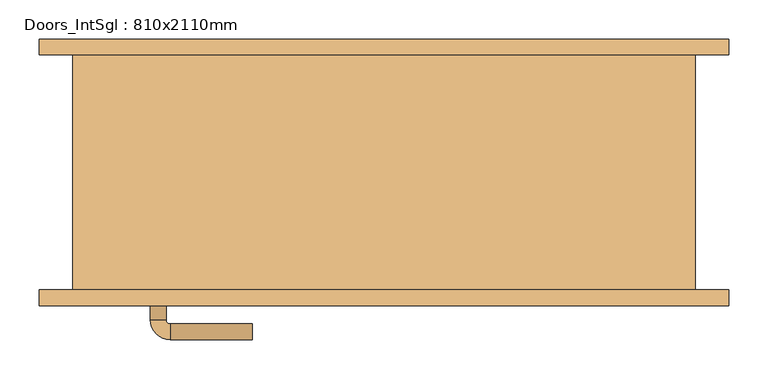
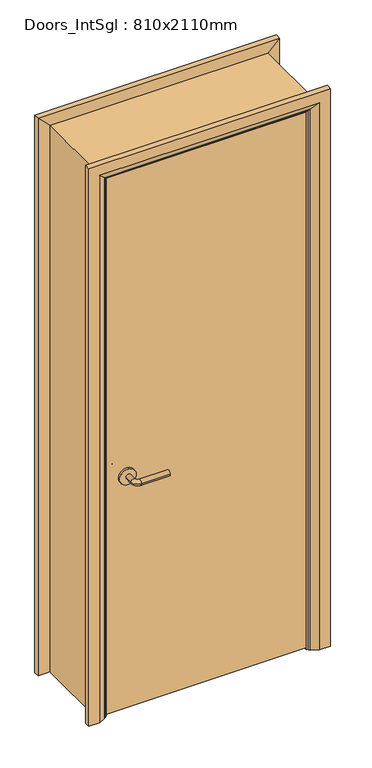
"""IFC4 building model written with IfcOpenShell, lengths in millimetres: door geometry, Doors_IntSgl : 810x2110mm."""

from ifc_helpers import new_model, si_unit, point, frame, frame_2d, origin, place, context, project, spatial, polyline, circle_curve, ellipse_curve, trimmed, segment, composite_curve, outline, extrude, faceted_brep, source, transform, mapped, element, save
from ifc_brep_helpers import plane_surface, cylinder_surface, revolved_surface, advanced_brep


def doors_intsgl_810x2110mm_8206dd41(model_context):
    return source(origin(), model_context, "Body", "SolidModel", [
        advanced_brep(
        [(-298.0, -104.0, 900.0), (-278.0, -104.0, 900.0), (-298.0, -74.0, 900.0), (-278.0, -74.0, 900.0), (-273.0, -69.0, 900.0), (-273.0, -49.0, 900.0), (-168.0, -49.0, 900.0), (-168.0, -69.0, 900.0)],
        [
            (0, 1, circle_curve(frame((-288.0, -104.0, 900.0), z_axis=(0.0, -1.0, 0.0), x_axis=(1.0, 0.0, 0.0)), 10.0)),
            (1, 0, circle_curve(frame((-288.0, -104.0, 900.0), z_axis=(0.0, -1.0, 0.0), x_axis=(1.0, 0.0, 0.0)), 10.0)),
            (0, 2),
            (2, 3, circle_curve(frame((-288.0, -74.0, 900.0), z_axis=(0.0, -1.0, 0.0), x_axis=(1.0, 0.0, 0.0)), 10.0)),
            (3, 1),
            (3, 2, circle_curve(frame((-288.0, -74.0, 900.0), z_axis=(0.0, -1.0, 0.0), x_axis=(1.0, 0.0, 0.0)), 10.0)),
            (4, 3, circle_curve(frame((-273.0, -74.0, 900.0), z_axis=(0.0, 0.0, 1.0), x_axis=(-1.0, 0.0, 0.0)), 5.0)),
            (2, 5, circle_curve(frame((-273.0, -74.0, 900.0), z_axis=(0.0, 0.0, -1.0), x_axis=(-1.0, 0.0, 0.0)), 25.0)),
            (5, 4, circle_curve(frame((-273.0, -59.0, 900.0), z_axis=(-1.0, 0.0, 0.0), x_axis=(0.0, -1.0, 0.0)), 10.0)),
            (4, 5, circle_curve(frame((-273.0, -59.0, 900.0), z_axis=(-1.0, 0.0, 0.0), x_axis=(0.0, -1.0, 0.0)), 10.0)),
            (6, 7, circle_curve(frame((-168.0, -59.0, 900.0), z_axis=(1.0, 0.0, 0.0), x_axis=(0.0, -1.0, 0.0)), 10.0)),
            (7, 6, circle_curve(frame((-168.0, -59.0, 900.0), z_axis=(1.0, 0.0, 0.0), x_axis=(0.0, -1.0, 0.0)), 10.0)),
            (5, 6),
            (7, 4),
        ],
        [
            plane_surface(frame((-288.0, -104.0, 900.0), z_axis=(0.0, -1.0, 0.0), x_axis=(0.0, 0.0, 1.0))),
            cylinder_surface(frame((-288.0, -104.0, 900.0), z_axis=(0.0, -1.0, 0.0), x_axis=(1.0, 0.0, 0.0)), 10.0),
            revolved_surface(trimmed(ellipse_curve(frame((-288.0, -74.0, 900.0), z_axis=(0.0, -1.0, 0.0), x_axis=(1.0, 0.0, 0.0)), 10.0, 10.0), [point((-298.0, -74.0, 900.0))], [point((-278.0, -74.0, 900.0))], True, "CARTESIAN"), (-273.0, -74.0, 900.0), (0.0, 0.0, -1.0)),
            revolved_surface(trimmed(ellipse_curve(frame((-288.0, -74.0, 900.0), z_axis=(0.0, -1.0, 0.0), x_axis=(1.0, 0.0, 0.0)), 10.0, 10.0), [point((-278.0, -74.0, 900.0))], [point((-298.0, -74.0, 900.0))], True, "CARTESIAN"), (-273.0, -74.0, 900.0), (0.0, 0.0, -1.0)),
            plane_surface(frame((-168.0, -59.0, 900.0), z_axis=(1.0, 0.0, 0.0), x_axis=(0.0, 0.0, 1.0))),
            cylinder_surface(frame((-273.0, -59.0, 900.0), z_axis=(-1.0, 0.0, 0.0), x_axis=(0.0, -1.0, 0.0)), 10.0),
        ],
        [
            (0, [[1, 2]]),
            (1, [[-1, 3, 4, 5]]),
            (1, [[-2, -5, 6, -3]]),
            (2, [[7, -4, 8, 9]]),
            (3, [[-8, -6, -7, 10]]),
            (4, [[11, 12]]),
            (5, [[-9, 13, -12, 14]]),
            (5, [[-10, -14, -11, -13]]),
        ],
    ),
        extrude(outline(composite_curve([segment(trimmed(circle_curve(frame_2d((900.0, -290.5)), 30.0), [point((900.0, -320.5))], [point((900.0, -260.5))], False, "CARTESIAN"), True, "CONTINUOUS"), segment(trimmed(circle_curve(frame_2d((900.0, -290.5)), 30.0), [point((900.0, -260.5))], [point((900.0, -320.5))], False, "CARTESIAN"), True, "CONTINUOUS")], self_intersect=False)), frame((0.0, -112.0, 0.0), z_axis=(0.0, 1.0, 0.0), x_axis=(0.0, 0.0, 1.0)), (0.0, 0.0, 1.0), 8.0),
        advanced_brep(
        [(-298.0, -158.0, 900.0), (-278.0, -158.0, 900.0), (-278.0, -188.0, 900.0), (-298.0, -188.0, 900.0), (-273.0, -193.0, 900.0), (-273.0, -213.0, 900.0), (-168.0, -213.0, 900.0), (-168.0, -193.0, 900.0)],
        [
            (0, 1, circle_curve(frame((-288.0, -158.0, 900.0), z_axis=(0.0, 1.0, 0.0), x_axis=(1.0, 0.0, 0.0)), 10.0)),
            (1, 0, circle_curve(frame((-288.0, -158.0, 900.0), z_axis=(0.0, 1.0, 0.0), x_axis=(1.0, 0.0, 0.0)), 10.0)),
            (1, 2),
            (2, 3, circle_curve(frame((-288.0, -188.0, 900.0), z_axis=(0.0, 1.0, 0.0), x_axis=(1.0, 0.0, 0.0)), 10.0)),
            (3, 0),
            (3, 2, circle_curve(frame((-288.0, -188.0, 900.0), z_axis=(0.0, 1.0, 0.0), x_axis=(1.0, 0.0, 0.0)), 10.0)),
            (4, 5, circle_curve(frame((-273.0, -203.0, 900.0), z_axis=(-1.0, 0.0, 0.0), x_axis=(0.0, 1.0, 0.0)), 10.0)),
            (5, 3, circle_curve(frame((-273.0, -188.0, 900.0), z_axis=(0.0, 0.0, -1.0), x_axis=(-1.0, 0.0, 0.0)), 25.0)),
            (2, 4, circle_curve(frame((-273.0, -188.0, 900.0), z_axis=(0.0, 0.0, 1.0), x_axis=(-1.0, 0.0, 0.0)), 5.0)),
            (5, 4, circle_curve(frame((-273.0, -203.0, 900.0), z_axis=(-1.0, 0.0, 0.0), x_axis=(0.0, 1.0, 0.0)), 10.0)),
            (6, 7, circle_curve(frame((-168.0, -203.0, 900.0), z_axis=(1.0, 0.0, 0.0), x_axis=(0.0, 1.0, 0.0)), 10.0)),
            (7, 6, circle_curve(frame((-168.0, -203.0, 900.0), z_axis=(1.0, 0.0, 0.0), x_axis=(0.0, 1.0, 0.0)), 10.0)),
            (4, 7),
            (6, 5),
        ],
        [
            plane_surface(frame((-288.0, -158.0, 900.0), z_axis=(0.0, 1.0, 0.0), x_axis=(0.0, 0.0, 1.0))),
            cylinder_surface(frame((-288.0, -158.0, 900.0), z_axis=(0.0, 1.0, 0.0), x_axis=(1.0, 0.0, 0.0)), 10.0),
            revolved_surface(trimmed(ellipse_curve(frame((-288.0, -188.0, 900.0), z_axis=(0.0, -1.0, 0.0), x_axis=(1.0, 0.0, 0.0)), 10.0, 10.0), [point((-298.0, -188.0, 900.0))], [point((-278.0, -188.0, 900.0))], True, "CARTESIAN"), (-273.0, -188.0, 900.0), (0.0, 0.0, -1.0)),
            revolved_surface(trimmed(ellipse_curve(frame((-288.0, -188.0, 900.0), z_axis=(0.0, -1.0, 0.0), x_axis=(1.0, 0.0, 0.0)), 10.0, 10.0), [point((-278.0, -188.0, 900.0))], [point((-298.0, -188.0, 900.0))], True, "CARTESIAN"), (-273.0, -188.0, 900.0), (0.0, 0.0, -1.0)),
            plane_surface(frame((-168.0, -203.0, 900.0), z_axis=(1.0, 0.0, 0.0), x_axis=(0.0, 0.0, 1.0))),
            cylinder_surface(frame((-273.0, -203.0, 900.0), z_axis=(-1.0, 0.0, 0.0), x_axis=(0.0, 1.0, 0.0)), 10.0),
        ],
        [
            (0, [[1, 2]]),
            (1, [[3, 4, 5, -2]]),
            (1, [[-5, 6, -3, -1]]),
            (2, [[7, 8, -4, 9]]),
            (3, [[10, -9, -6, -8]]),
            (4, [[11, 12]]),
            (5, [[13, -11, 14, -7]]),
            (5, [[-14, -12, -13, -10]]),
        ],
    ),
        extrude(outline(composite_curve([segment(trimmed(circle_curve(frame_2d((900.0, -290.5)), 30.0), [point((900.0, -320.5))], [point((900.0, -260.5))], False, "CARTESIAN"), True, "CONTINUOUS"), segment(trimmed(circle_curve(frame_2d((900.0, -290.5)), 30.0), [point((900.0, -260.5))], [point((900.0, -320.5))], False, "CARTESIAN"), True, "CONTINUOUS")], self_intersect=False)), frame((0.0, -158.0, 0.0), z_axis=(0.0, 1.0, 0.0), x_axis=(0.0, 0.0, 1.0)), (0.0, 0.0, 1.0), 8.0),
        extrude(outline(polyline([(363.0, -112.0), (363.0, -150.0), (-363.0, -150.0), (-363.0, -112.0), (363.0, -112.0)])), frame((0.0, 0.0, 8.0), z_axis=(0.0, 0.0, 1.0), x_axis=(1.0, 0.0, 0.0)), (0.0, 0.0, 1.0), 2060.0),
        advanced_brep(
        [(440.0, -170.0, 0.0), (400.0, -170.0, 0.0), (374.0, -156.0, 0.0), (370.0, -150.0, 0.0), (440.0, -150.0, 0.0), (440.0, -150.0, 2145.0), (440.0, -170.0, 2145.0), (370.0, -150.0, 2075.0), (-370.0, -150.0, 2075.0), (-370.0, -150.0, 0.0), (-440.0, -150.0, 0.0), (-440.0, -150.0, 2145.0), (374.0, -156.0, 2079.0), (400.0, -170.0, 2105.0), (-440.0, -170.0, 2145.0), (-440.0, -170.0, 0.0), (-400.0, -170.0, 0.0), (-400.0, -170.0, 2105.0), (-374.0, -156.0, 2079.0), (-374.0, -156.0, 0.0)],
        [
            (0, 1),
            (1, 2),
            (2, 3, circle_curve(frame((378.0, -149.0, 0.0), z_axis=(0.0, 0.0, -1.0), x_axis=(1.0, 0.0, 0.0)), 8.0622577)),
            (3, 4),
            (4, 0),
            (4, 5),
            (5, 6),
            (6, 0),
            (3, 7),
            (7, 8),
            (8, 9),
            (9, 10),
            (10, 11),
            (11, 5),
            (2, 12),
            (12, 7, ellipse_curve(frame((378.0, -149.0, 2083.0), z_axis=(0.7071067811865475, 0.0, -0.7071067811865475), x_axis=(-0.7071067811865474, 0.0, -0.7071067811865476)), 11.4017543, 8.0622577)),
            (1, 13),
            (13, 12),
            (6, 14),
            (14, 15),
            (15, 16),
            (16, 17),
            (17, 13),
            (11, 14),
            (12, 18),
            (18, 8, ellipse_curve(frame((-378.0, -149.0, 2083.0), z_axis=(0.7071067811865475, 0.0, 0.7071067811865475), x_axis=(0.7071067811865476, 0.0, -0.7071067811865474)), 11.4017543, 8.0622577)),
            (17, 18),
            (15, 10),
            (9, 19, circle_curve(frame((-378.0, -149.0, 0.0), z_axis=(0.0, 0.0, -1.0), x_axis=(-1.0, 0.0, 0.0)), 8.0622577)),
            (19, 16),
            (18, 19),
        ],
        [
            plane_surface(frame((370.0, -150.0, 0.0), z_axis=(0.0, 0.0, -1.0), x_axis=(0.0, 1.0, 0.0))),
            plane_surface(frame((440.0, -170.0, 0.0), z_axis=(1.0, 0.0, 0.0), x_axis=(0.0, 0.0, 1.0))),
            plane_surface(frame((440.0, -150.0, 0.0), z_axis=(0.0, 1.0, 0.0), x_axis=(0.0, 0.0, 1.0))),
            cylinder_surface(frame((378.0, -149.0, 0.0), z_axis=(0.0, 0.0, -1.0), x_axis=(1.0, 0.0, 0.0)), 8.0622577),
            plane_surface(frame((374.0, -156.0, 0.0), z_axis=(-0.4740998230350126, -0.880471099922178, 0.0), x_axis=(0.0, 0.0, 1.0))),
            plane_surface(frame((400.0, -170.0, 0.0), z_axis=(0.0, -1.0, 0.0), x_axis=(0.0, 0.0, 1.0))),
            plane_surface(frame((440.0, -170.0, 2145.0), z_axis=(0.0, 0.0, 1.0), x_axis=(-1.0, 0.0, 0.0))),
            cylinder_surface(frame((370.0, -149.0, 2083.0), z_axis=(1.0, 0.0, 0.0), x_axis=(0.0, 0.0, 1.0)), 8.0622577),
            plane_surface(frame((374.0, -156.0, 2079.0), z_axis=(0.0, -0.8804710999221764, -0.4740998230350154), x_axis=(-1.0, 0.0, 0.0))),
            plane_surface(frame((-370.0, -150.0, 0.0), z_axis=(0.0, 0.0, -1.0), x_axis=(0.0, 1.0, 0.0))),
            plane_surface(frame((-440.0, -170.0, 2145.0), z_axis=(-1.0, 0.0, 0.0), x_axis=(0.0, 0.0, -1.0))),
            cylinder_surface(frame((-378.0, -149.0, 2075.0), z_axis=(0.0, 0.0, 1.0), x_axis=(-1.0, 0.0, 0.0)), 8.0622577),
            plane_surface(frame((-374.0, -156.0, 2079.0), z_axis=(0.47409982303501824, -0.8804710999221749, 0.0), x_axis=(0.0, 0.0, -1.0))),
        ],
        [
            (0, [[1, 2, 3, 4, 5]]),
            (1, [[6, 7, 8, -5]]),
            (2, [[9, 10, 11, 12, 13, 14, -6, -4]]),
            (3, [[15, 16, -9, -3]]),
            (4, [[17, 18, -15, -2]]),
            (5, [[-8, 19, 20, 21, 22, 23, -17, -1]]),
            (6, [[-14, 24, -19, -7]]),
            (7, [[25, 26, -10, -16]]),
            (8, [[-23, 27, -25, -18]]),
            (9, [[28, -12, 29, 30, -21]]),
            (10, [[-13, -28, -20, -24]]),
            (11, [[31, -29, -11, -26]]),
            (12, [[-22, -30, -31, -27]]),
        ],
    ),
        extrude(outline(polyline([(0.0, -346.0), (2051.0, -346.0), (2051.0, 346.0), (0.0, 346.0), (0.0, 365.0), (2070.0, 365.0), (2070.0, -365.0), (0.0, -365.0), (0.0, -346.0)])), frame((0.0, -110.0, 0.0), z_axis=(0.0, 1.0, 0.0), x_axis=(0.0, 0.0, 1.0)), (0.0, 0.0, 1.0), 32.0),
        advanced_brep(
        [(-440.0, 170.0, 0.0), (-400.0, 170.0, 0.0), (-374.0, 156.0, 0.0), (-370.0, 150.0, 0.0), (-440.0, 150.0, 0.0), (-440.0, 150.0, 2145.0), (-440.0, 170.0, 2145.0), (-370.0, 150.0, 2075.0), (-374.0, 156.0, 2079.0), (-400.0, 170.0, 2105.0), (440.0, 150.0, 2145.0), (440.0, 170.0, 2145.0), (370.0, 150.0, 2075.0), (374.0, 156.0, 2079.0), (400.0, 170.0, 2105.0), (440.0, 170.0, 0.0), (440.0, 150.0, 0.0), (370.0, 150.0, 0.0), (374.0, 156.0, 0.0), (400.0, 170.0, 0.0)],
        [
            (0, 1),
            (1, 2),
            (2, 3, circle_curve(frame((-378.0, 149.0, 0.0), z_axis=(0.0, 0.0, -1.0), x_axis=(-1.0, 0.0, 0.0)), 8.0622577)),
            (3, 4),
            (4, 0),
            (4, 5),
            (5, 6),
            (6, 0),
            (3, 7),
            (7, 5),
            (2, 8),
            (8, 7, ellipse_curve(frame((-378.0, 149.0, 2083.0), z_axis=(-0.7071067811865475, 0.0, -0.7071067811865475), x_axis=(0.7071067811865474, 0.0, -0.7071067811865476)), 11.4017543, 8.0622577)),
            (1, 9),
            (9, 8),
            (6, 9),
            (5, 10),
            (10, 11),
            (11, 6),
            (7, 12),
            (12, 10),
            (8, 13),
            (13, 12, ellipse_curve(frame((378.0, 149.0, 2083.0), z_axis=(-0.7071067811865475, 0.0, 0.7071067811865475), x_axis=(-0.7071067811865476, 0.0, -0.7071067811865474)), 11.4017543, 8.0622577)),
            (9, 14),
            (14, 13),
            (11, 14),
            (15, 16),
            (16, 17),
            (17, 18, circle_curve(frame((378.0, 149.0, 0.0), z_axis=(0.0, 0.0, -1.0), x_axis=(1.0, 0.0, 0.0)), 8.0622577)),
            (18, 19),
            (19, 15),
            (10, 16),
            (15, 11),
            (12, 17),
            (13, 18),
            (14, 19),
        ],
        [
            plane_surface(frame((-370.0, 222.8010989, 0.0), z_axis=(0.0, 0.0, -1.0), x_axis=(1.0, 0.0, 0.0))),
            plane_surface(frame((-440.0, 170.0, 0.0), z_axis=(-1.0, 0.0, 0.0), x_axis=(0.0, 0.0, 1.0))),
            plane_surface(frame((-440.0, 150.0, 0.0), z_axis=(0.0, -1.0, 0.0), x_axis=(0.0, 0.0, 1.0))),
            cylinder_surface(frame((-378.0, 149.0, 0.0), z_axis=(0.0, 0.0, -1.0), x_axis=(-1.0, 0.0, 0.0)), 8.0622577),
            plane_surface(frame((-374.0, 156.0, 0.0), z_axis=(0.4740998230350183, 0.8804710999221749, 0.0), x_axis=(0.0, 0.0, 1.0))),
            plane_surface(frame((-400.0, 170.0, 0.0), z_axis=(0.0, 1.0, 0.0), x_axis=(0.0, 0.0, 1.0))),
            plane_surface(frame((-440.0, 170.0, 2145.0), z_axis=(0.0, 0.0, 1.0), x_axis=(1.0, 0.0, 0.0))),
            plane_surface(frame((-440.0, 150.0, 2145.0), z_axis=(0.0, -1.0, 0.0), x_axis=(1.0, 0.0, 0.0))),
            cylinder_surface(frame((-370.0, 149.0, 2083.0), z_axis=(-1.0, 0.0, 0.0), x_axis=(0.0, 0.0, 1.0)), 8.0622577),
            plane_surface(frame((-374.0, 156.0, 2079.0), z_axis=(0.0, 0.8804710999221749, -0.4740998230350183), x_axis=(1.0, 0.0, 0.0))),
            plane_surface(frame((-400.0, 170.0, 2105.0), z_axis=(0.0, 1.0, 0.0), x_axis=(1.0, 0.0, 0.0))),
            plane_surface(frame((370.0, 222.8010989, 0.0), z_axis=(0.0, 0.0, -1.0), x_axis=(-1.0, 0.0, 0.0))),
            plane_surface(frame((440.0, 170.0, 2145.0), z_axis=(1.0, 0.0, 0.0), x_axis=(0.0, 0.0, -1.0))),
            plane_surface(frame((440.0, 150.0, 2145.0), z_axis=(0.0, -1.0, 0.0), x_axis=(0.0, 0.0, -1.0))),
            cylinder_surface(frame((378.0, 149.0, 2075.0), z_axis=(0.0, 0.0, 1.0), x_axis=(1.0, 0.0, 0.0)), 8.0622577),
            plane_surface(frame((374.0, 156.0, 2079.0), z_axis=(-0.4740998230350183, 0.8804710999221749, 0.0), x_axis=(0.0, 0.0, -1.0))),
            plane_surface(frame((400.0, 170.0, 2105.0), z_axis=(0.0, 1.0, 0.0), x_axis=(0.0, 0.0, -1.0))),
        ],
        [
            (0, [[1, 2, 3, 4, 5]]),
            (1, [[6, 7, 8, -5]]),
            (2, [[9, 10, -6, -4]]),
            (3, [[11, 12, -9, -3]]),
            (4, [[13, 14, -11, -2]]),
            (5, [[-8, 15, -13, -1]]),
            (6, [[16, 17, 18, -7]]),
            (7, [[19, 20, -16, -10]]),
            (8, [[21, 22, -19, -12]]),
            (9, [[23, 24, -21, -14]]),
            (10, [[-18, 25, -23, -15]]),
            (11, [[26, 27, 28, 29, 30]]),
            (12, [[31, -26, 32, -17]]),
            (13, [[33, -27, -31, -20]]),
            (14, [[34, -28, -33, -22]]),
            (15, [[35, -29, -34, -24]]),
            (16, [[-32, -30, -35, -25]]),
        ],
    ),
        faceted_brep([(-365.0, -150.0, 0.0), (-397.0, -150.0, 0.0), (-397.0, 150.0, 0.0), (-365.0, 150.0, 0.0), (-365.0, 150.0, 2070.0), (-365.0, -150.0, 2070.0), (-397.0, 150.0, 2102.0), (-397.0, -150.0, 2102.0), (365.0, 150.0, 2070.0), (365.0, -150.0, 2070.0), (397.0, 150.0, 2102.0), (397.0, -150.0, 2102.0), (365.0, -150.0, 0.0), (365.0, 150.0, 0.0), (397.0, 150.0, 0.0), (397.0, -150.0, 0.0)], [[[0, 1, 2, 3]], [[3, 4, 5, 0]], [[2, 6, 4, 3]], [[1, 7, 6, 2]], [[0, 5, 7, 1]], [[4, 8, 9, 5]], [[6, 10, 8, 4]], [[7, 11, 10, 6]], [[5, 9, 11, 7]], [[12, 13, 14, 15]], [[8, 13, 12, 9]], [[10, 14, 13, 8]], [[11, 15, 14, 10]], [[9, 12, 15, 11]]]),
    ])


if __name__ == "__main__":
    model = new_model("IFC4")
    model_context = context("Model", 3, world=origin())
    ifc_project = project(units=[si_unit("LENGTHUNIT", "METRE", prefix="MILLI")], contexts=[model_context])
    site = spatial("IfcSite", under=ifc_project)
    building = spatial("IfcBuilding", under=site)
    placement = place(None, origin())
    doors_intsgl_810x2110mm_shape = doors_intsgl_810x2110mm_8206dd41(model_context)
    element("IfcDoor", 1, ObjectType="Doors_IntSgl : 810x2110mm", at=placement, inside=building, context=model_context, shape_type="MappedRepresentation", body=[
        mapped(doors_intsgl_810x2110mm_shape, transform((0.0, 0.0, 0.0), x_axis=(1.0, 0.0, 0.0), y_axis=(0.0, 1.0, 0.0), z_axis=(0.0, 0.0, 1.0))),
    ])
    save(model, "model.ifc")

# Revit data of these elements
# Type "Doors_IntSgl : 810x2110mm"
#   Construction Type Id = "MDOOR"
#   Type Mark = "42"
#   Type Comments = "Internal Single"
#   Operation = "SingleSwingRight"
#   Manufacturer = "Revit"
#   Keynote = "L20"
#   Description = "Internal Single Door"
#   Analytic Construction = "Metal"
#   UnderCut = 8 mm
#   Tolerance = 2 mm
#   Thickness = 38 mm
#   Thermal Resistance (R) = 0.270117 (m²·K)/W
#   Structural Tolerance = 8 mm
#   StopDepth = 32 mm
#   Stop Thickness = 19 mm
#   Rough Width = 810 mm
#   Rough Height = 2110 mm
#   Height to Top Lock Rail = 1000 mm
#   Heat Transfer Coefficient (U) = 3.7021 W/(m²·K)
#   Handle Z Distance = 900 mm
#   Handle X Distance = 75 mm
#   Frame Thickness = 32 mm
#   Door Panel Width = 726 mm
#   Door Panel Thickness = 38 mm
#   Door Panel Offset = 0 mm
#   Height = 2110 mm
#   Width = 810 mm
#   Door Panel Height = 2060 mm
#   Architrave Setback = 5 mm
#   Define Thermal Properties by = 1
#   Vis - Ironmongery = yes
#   Material Ironmongery = Door - Handle
#   Material Frame = Door - Frame/Mullion (1)
#   Material Door = Door - Panel
#   Material Architrave = Door - Architrave
#   Visual Light Transmittance = 0
#   Solar Heat Gain Coefficient = 0
#   Function = (empty or 0)
#   Wall Closure = (empty or 0)
# Element 1 (IfcDoor, "Doors_IntSgl : 810x2110mm")
#   Materials on its faces: "Door - Architrave", "Door - Handle", "Door - Frame/Mullion (1)", "Door - Panel"
# Materials
#   "Door - Handle": colour RGB 0 0 0, transparency 0, Keynote = "P21", Cost = 0
#   "Door - Frame/Mullion (1)": class "Wood", colour RGB 212 179 113, transparency 0, Keynote = "L20", Cost = 0
#   "Door - Panel": class "Wood", colour RGB 210 159 95, transparency 0, Keynote = "L20", Cost = 0
#   "Door - Architrave": class "Wood", colour RGB 154 90 5, transparency 0, Keynote = "P20", Cost = 0
